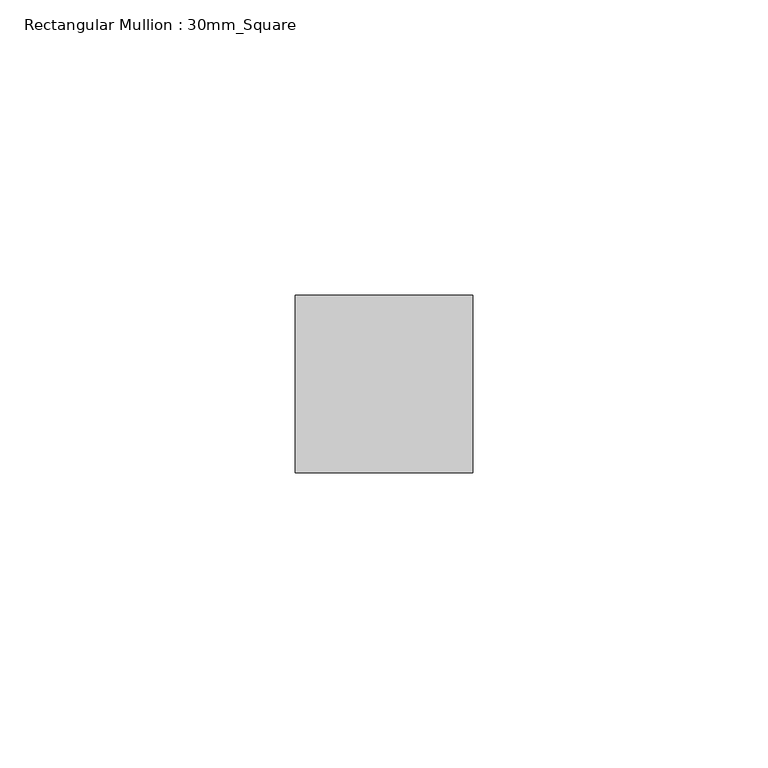
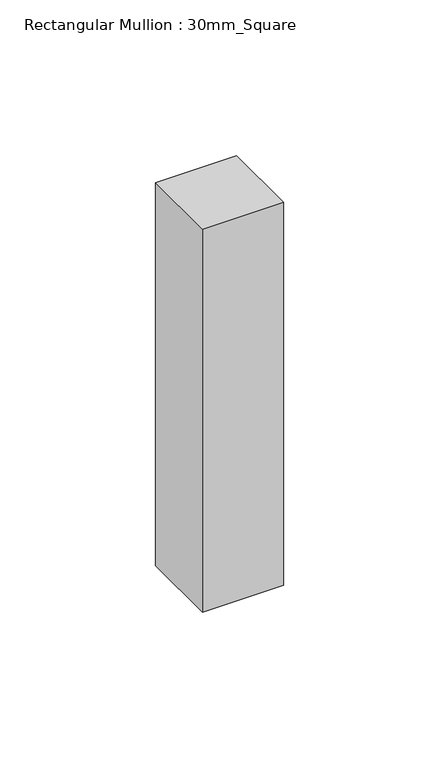
"""IFC4 building model written with IfcOpenShell, lengths in millimetres: member geometry, Rectangular Mullion : 30mm_Square."""

from ifc_helpers import new_model, si_unit, frame, origin, place, context, project, spatial, polyline, outline, extrude, source, transform, mapped, element, save


def rectangular_mullion_30mm_square_e994106c(model_context):
    return source(origin(), model_context, "Body", "SweptSolid", [
        extrude(outline(polyline([(15.0, 15.0), (15.0, -15.0), (-15.0, -15.0), (-15.0, 15.0), (15.0, 15.0)])), frame((0.0, 0.0, -150.0429688), z_axis=(0.0, 0.0, 1.0), x_axis=(1.0, 0.0, 0.0)), (0.0, 0.0, 1.0), 150.0429688),
    ])


if __name__ == "__main__":
    model = new_model("IFC4")
    model_context = context("Model", 3, world=origin())
    ifc_project = project(units=[si_unit("LENGTHUNIT", "METRE", prefix="MILLI")], contexts=[model_context])
    site = spatial("IfcSite", under=ifc_project)
    building = spatial("IfcBuilding", under=site)
    placement = place(None, origin())
    rectangular_mullion_30mm_square_shape = rectangular_mullion_30mm_square_e994106c(model_context)
    element("IfcMember", 1, ObjectType="Rectangular Mullion : 30mm_Square", at=placement, inside=building, context=model_context, shape_type="MappedRepresentation", body=[
        mapped(rectangular_mullion_30mm_square_shape, transform((0.0, 0.0, 0.0), x_axis=(1.0, 0.0, 0.0), y_axis=(0.0, 1.0, 0.0), z_axis=(0.0, 0.0, 1.0))),
    ])
    save(model, "model.ifc")

# Revit data of these elements
# Type "Rectangular Mullion : 30mm_Square"
#   Keynote = "H11"
#   built-in parameter 1007304 = 0.0984252 (stored number, unit not read)
#   built-in parameter 1007301 = 0.0492126 (stored number, unit not read)
#   built-in parameter 1007300 = 0.0492126 (stored number, unit not read)
# Element 1 (IfcMember, "Rectangular Mullion : 30mm_Square")
#   Materials on its faces: "Aluminium"
# Materials
#   "Aluminium": class "Metal", colour RGB 247 247 247, transparency 0, Description = "Aluminium 6061", Cost = 0
